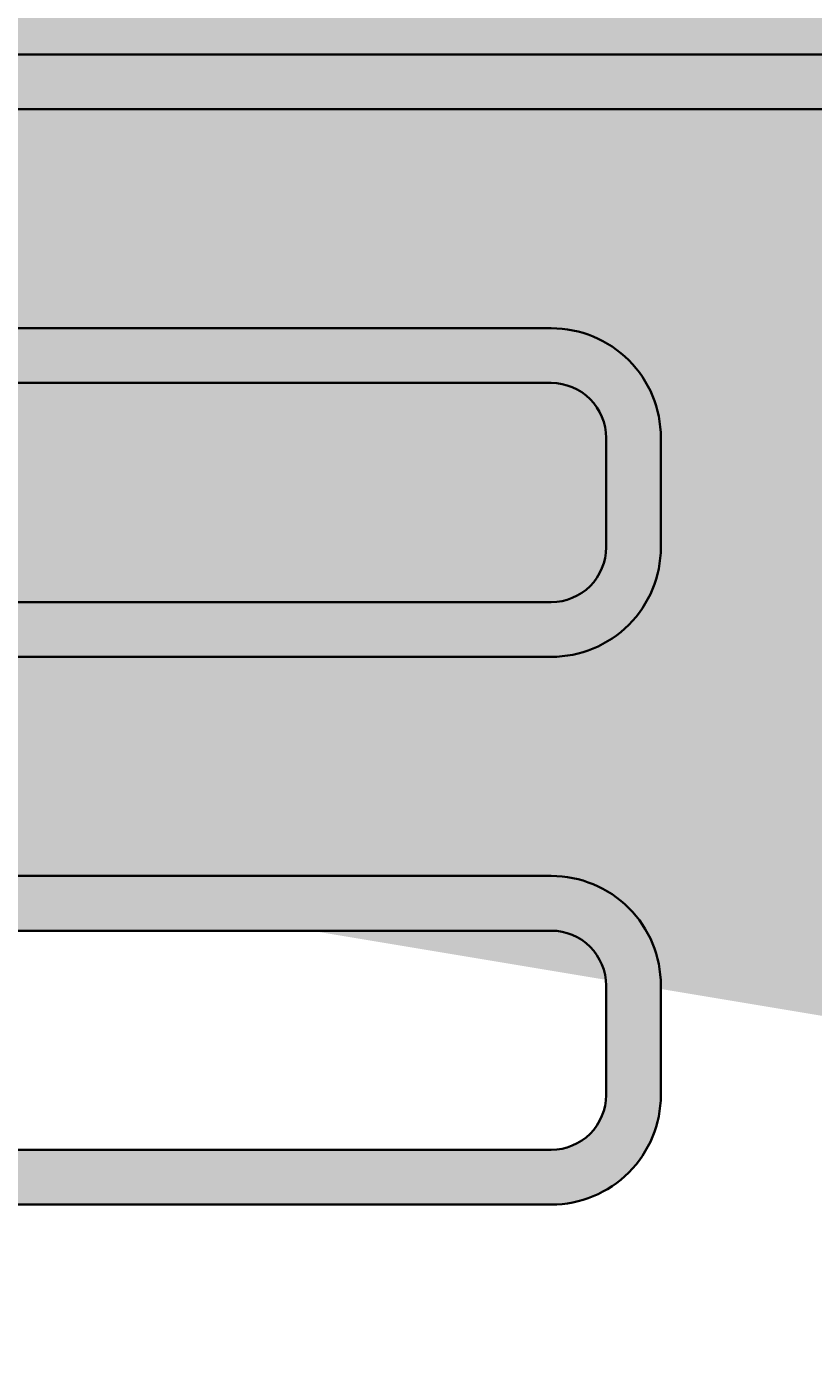
# Model space of a CAD drawing. Units: millimetres. Extents: x -22994 to 29398, y -19990 to 20176.
# Tile 40 of 135: x 169 to 183, y 54 to 78. Entities that reach past the tile are written whole.
import ezdxf

# ---------------------------------------------------------------- set-up
doc = ezdxf.new("R2010")
doc.units = ezdxf.units.MM
doc.header["$MEASUREMENT"] = 0
for name, color, linetype, lineweight in [('M-DIMS', 2, 'Continuous', 18), ('M-EQPM-PATT', 7, 'Continuous', 18), ('M-PIPE', 7, 'Continuous', 35)]:
    doc.layers.add(name, color=color, linetype=linetype, lineweight=lineweight)
doc.styles.get("Standard").update_dxf_attribs({"font": 'arial.ttf'})
doc.dimstyles.get("Standard").update_dxf_attribs({"dimtxt": 0.18, "dimasz": 10000, "dimexe": 0.18, "dimexo": 0.0625, "dimgap": 0.09, "dimtad": 0, "dimtih": 1, "dimtoh": 1, "dimdec": 0, "dimzin": 0, "dimdsep": 46, "dimtxsty": 'Standard', "dimcen": 0.09, "dimadec": 0, "dimazin": 0, "dimtfac": 1, "dimtdec": 0, "dimtofl": 0, "dimtmove": 0, "dimatfit": 3, "dimfxl": 1, "dimtolj": 1, "dimtzin": 0, "dimlwd": 30, "dimarcsym": 0})

# ---------------------------------------------------------------- blocks, each defined once
blk = doc.blocks.new('*D2')
at = {"layer": 'Defpoints', "color": 0, "transparency": 16777216}
for p in [(6.677, 10.271), (290.852, 10.271), (290.852, -5.079)]:
    blk.add_point(p, dxfattribs=at)
at = {"layer": 'M-DIMS', "color": 0, "lineweight": -2, "transparency": 16777216}
for p, q in [((6.677, 10.209), (6.677, -5.259)), ((290.852, 10.209), (290.852, -5.259))]:
    blk.add_line(p, q, dxfattribs=at)
at = {"layer": 'M-DIMS', "color": 0, "lineweight": 30, "transparency": 16777216}
for p, q in [((-9993.323, -5.079), (-19993.323, -5.079)), ((10290.852, -5.079), (20290.852, -5.079))]:
    blk.add_line(p, q, dxfattribs=at)
at = {"layer": 'M-DIMS', "color": 0, "transparency": 16777216}
for points in [[(-9993.323, 1661.588), (-9993.323, -1671.745), (6.677, -5.079)], [(10290.852, 1661.588), (10290.852, -1671.745), (290.852, -5.079)]]:
    blk.add_solid(points, dxfattribs=at)
at = {"layer": 'M-DIMS', "color": 0, "transparency": 16777216, "insert": (148.765, -5.079), "char_height": 0.18, "attachment_point": 5}
blk.add_mtext('\\A1;284.2', dxfattribs=at)
blk = doc.blocks.new('*D3')
at = {"layer": 'Defpoints', "color": 0, "transparency": 16777216}
for p in [(110.265, 204.165), (110.265, 176.366), (95.833, 127.967)]:
    blk.add_point(p, dxfattribs=at)
at = {"layer": 'M-DIMS', "color": 0, "lineweight": -2, "transparency": 16777216}
for p, q in [((95.833, 128.03), (95.833, 204.345)), ((110.265, 176.429), (110.265, 204.345))]:
    blk.add_line(p, q, dxfattribs=at)
at = {"layer": 'M-DIMS', "color": 0, "lineweight": 30, "transparency": 16777216}
for p, q in [((-9904.167, 204.165), (-19904.167, 204.165)), ((10110.265, 204.165), (20110.265, 204.165))]:
    blk.add_line(p, q, dxfattribs=at)
at = {"layer": 'M-DIMS', "color": 0, "transparency": 16777216}
for points in [[(-9904.167, 1870.832), (-9904.167, -1462.501), (95.833, 204.165)], [(10110.265, 1870.832), (10110.265, -1462.501), (110.265, 204.165)]]:
    blk.add_solid(points, dxfattribs=at)
at = {"layer": 'M-DIMS', "color": 0, "transparency": 16777216, "insert": (103.049, 204.165), "char_height": 0.18, "attachment_point": 5}
blk.add_mtext('\\A1;14.432', dxfattribs=at)
blk = doc.blocks.new('*D4')
at = {"layer": 'Defpoints', "color": 0, "transparency": 16777216}
for p in [(116.265, 204.165), (110.265, 176.366), (116.265, 176.366)]:
    blk.add_point(p, dxfattribs=at)
at = {"layer": 'M-DIMS', "color": 0, "lineweight": -2, "transparency": 16777216}
for p, q in [((110.265, 176.429), (110.265, 204.345)), ((116.265, 176.429), (116.265, 204.345))]:
    blk.add_line(p, q, dxfattribs=at)
at = {"layer": 'M-DIMS', "color": 0, "lineweight": 30, "transparency": 16777216}
for p, q in [((-9889.735, 204.165), (-19889.735, 204.165)), ((10116.265, 204.165), (20116.265, 204.165))]:
    blk.add_line(p, q, dxfattribs=at)
at = {"layer": 'M-DIMS', "color": 0, "transparency": 16777216}
for points in [[(-9889.735, 1870.832), (-9889.735, -1462.501), (110.265, 204.165)], [(10116.265, 1870.832), (10116.265, -1462.501), (116.265, 204.165)]]:
    blk.add_solid(points, dxfattribs=at)
at = {"layer": 'M-DIMS', "color": 0, "transparency": 16777216, "insert": (113.265, 204.165), "char_height": 0.18, "attachment_point": 5}
blk.add_mtext('\\A1;6', dxfattribs=at)
blk = doc.blocks.new('*D5')
at = {"layer": 'Defpoints', "color": 0, "transparency": 16777216}
for p in [(181.265, 204.165), (116.265, 176.366), (181.265, 176.366)]:
    blk.add_point(p, dxfattribs=at)
at = {"layer": 'M-DIMS', "color": 0, "lineweight": -2, "transparency": 16777216}
for p, q in [((116.265, 176.429), (116.265, 204.345)), ((181.265, 176.429), (181.265, 204.345))]:
    blk.add_line(p, q, dxfattribs=at)
at = {"layer": 'M-DIMS', "color": 0, "lineweight": 30, "transparency": 16777216}
for p, q in [((-9883.735, 204.165), (-19883.735, 204.165)), ((10181.265, 204.165), (20181.265, 204.165))]:
    blk.add_line(p, q, dxfattribs=at)
at = {"layer": 'M-DIMS', "color": 0, "transparency": 16777216}
for points in [[(-9883.735, 1870.832), (-9883.735, -1462.501), (116.265, 204.165)], [(10181.265, 1870.832), (10181.265, -1462.501), (181.265, 204.165)]]:
    blk.add_solid(points, dxfattribs=at)
at = {"layer": 'M-DIMS', "color": 0, "transparency": 16777216, "insert": (148.765, 204.165), "char_height": 0.18, "attachment_point": 5}
blk.add_mtext('\\A1;65', dxfattribs=at)
blk = doc.blocks.new('*D6')
at = {"layer": 'Defpoints', "color": 0, "transparency": 16777216}
for p in [(187.265, 204.165), (181.265, 176.366), (187.265, 176.366)]:
    blk.add_point(p, dxfattribs=at)
at = {"layer": 'M-DIMS', "color": 0, "lineweight": -2, "transparency": 16777216}
for p, q in [((181.265, 176.429), (181.265, 204.345)), ((187.265, 176.429), (187.265, 204.345))]:
    blk.add_line(p, q, dxfattribs=at)
at = {"layer": 'M-DIMS', "color": 0, "lineweight": 30, "transparency": 16777216}
for p, q in [((-9818.735, 204.165), (-19818.735, 204.165)), ((10187.265, 204.165), (20187.265, 204.165))]:
    blk.add_line(p, q, dxfattribs=at)
at = {"layer": 'M-DIMS', "color": 0, "transparency": 16777216}
for points in [[(-9818.735, 1870.832), (-9818.735, -1462.501), (181.265, 204.165)], [(10187.265, 1870.832), (10187.265, -1462.501), (187.265, 204.165)]]:
    blk.add_solid(points, dxfattribs=at)
at = {"layer": 'M-DIMS', "color": 0, "transparency": 16777216, "insert": (184.265, 204.165), "char_height": 0.18, "attachment_point": 5}
blk.add_mtext('\\A1;6', dxfattribs=at)
blk = doc.blocks.new('*D7')
at = {"layer": 'Defpoints', "color": 0, "transparency": 16777216}
for p in [(201.697, 204.165), (187.265, 176.366), (201.697, 127.967)]:
    blk.add_point(p, dxfattribs=at)
at = {"layer": 'M-DIMS', "color": 0, "lineweight": -2, "transparency": 16777216}
for p, q in [((187.265, 176.429), (187.265, 204.345)), ((201.697, 128.03), (201.697, 204.345))]:
    blk.add_line(p, q, dxfattribs=at)
at = {"layer": 'M-DIMS', "color": 0, "lineweight": 30, "transparency": 16777216}
for p, q in [((-9812.735, 204.165), (-19812.735, 204.165)), ((10201.697, 204.165), (20201.697, 204.165))]:
    blk.add_line(p, q, dxfattribs=at)
at = {"layer": 'M-DIMS', "color": 0, "transparency": 16777216}
for points in [[(-9812.735, 1870.832), (-9812.735, -1462.501), (187.265, 204.165)], [(10201.697, 1870.832), (10201.697, -1462.501), (201.697, 204.165)]]:
    blk.add_solid(points, dxfattribs=at)
at = {"layer": 'M-DIMS', "color": 0, "transparency": 16777216, "insert": (194.481, 204.165), "char_height": 0.18, "attachment_point": 5}
blk.add_mtext('\\A1;14.432', dxfattribs=at)
blk = doc.blocks.new('*D8')
at = {"layer": 'Defpoints', "color": 0, "transparency": 16777216}
for p in [(227.648, 204.165), (227.648, 146.73), (201.697, 127.967)]:
    blk.add_point(p, dxfattribs=at)
at = {"layer": 'M-DIMS', "color": 0, "lineweight": -2, "transparency": 16777216}
for p, q in [((201.697, 128.03), (201.697, 204.345)), ((227.648, 146.792), (227.648, 204.345))]:
    blk.add_line(p, q, dxfattribs=at)
at = {"layer": 'M-DIMS', "color": 0, "lineweight": 30, "transparency": 16777216}
for p, q in [((-9798.303, 204.165), (-19798.303, 204.165)), ((10227.648, 204.165), (20227.648, 204.165))]:
    blk.add_line(p, q, dxfattribs=at)
at = {"layer": 'M-DIMS', "color": 0, "transparency": 16777216}
for points in [[(-9798.303, 1870.832), (-9798.303, -1462.501), (201.697, 204.165)], [(10227.648, 1870.832), (10227.648, -1462.501), (227.648, 204.165)]]:
    blk.add_solid(points, dxfattribs=at)
at = {"layer": 'M-DIMS', "color": 0, "transparency": 16777216, "insert": (214.673, 204.165), "char_height": 0.18, "attachment_point": 5}
blk.add_mtext('\\A1;25.95', dxfattribs=at)
blk = doc.blocks.new('*D9')
at = {"layer": 'Defpoints', "color": 0, "transparency": 16777216}
for p in [(187.265, 176.366), (306.202, 176.366), (290.852, 10.271)]:
    blk.add_point(p, dxfattribs=at)
at = {"layer": 'M-DIMS', "color": 0, "lineweight": 30, "transparency": 16777216}
for p, q in [((306.202, 10176.366), (306.202, 20176.366)), ((306.202, -9989.729), (306.202, -19989.729))]:
    blk.add_line(p, q, dxfattribs=at)
at = {"layer": 'M-DIMS', "color": 0, "lineweight": -2, "transparency": 16777216}
for p, q in [((187.327, 176.366), (306.382, 176.366)), ((290.915, 10.271), (306.382, 10.271))]:
    blk.add_line(p, q, dxfattribs=at)
at = {"layer": 'M-DIMS', "color": 0, "transparency": 16777216}
for points in [[(-1360.465, 10176.366), (1972.869, 10176.366), (306.202, 176.366)], [(-1360.465, -9989.729), (1972.869, -9989.729), (306.202, 10.271)]]:
    blk.add_solid(points, dxfattribs=at)
at = {"layer": 'M-DIMS', "color": 0, "transparency": 16777216, "insert": (306.202, 93.319), "char_height": 0.18, "attachment_point": 5}
blk.add_mtext('\\A1;166.1', dxfattribs=at)
blk = doc.blocks.new('*D10')
at = {"layer": 'Defpoints', "color": 0, "transparency": 16777216}
for p in [(125.65, 136.071), (133.346, 136.071), (133.346, -5.079)]:
    blk.add_point(p, dxfattribs=at)
at = {"layer": 'M-DIMS', "color": 0, "lineweight": -2, "transparency": 16777216}
for p, q in [((125.65, 136.009), (125.65, -5.259)), ((133.346, 136.009), (133.346, -5.259))]:
    blk.add_line(p, q, dxfattribs=at)
at = {"layer": 'M-DIMS', "color": 0, "lineweight": 30, "transparency": 16777216}
for p, q in [((-9874.35, -5.079), (-19874.35, -5.079)), ((10133.346, -5.079), (20133.346, -5.079))]:
    blk.add_line(p, q, dxfattribs=at)
at = {"layer": 'M-DIMS', "color": 0, "transparency": 16777216}
for points in [[(-9874.35, 1661.588), (-9874.35, -1671.745), (125.65, -5.079)], [(10133.346, 1661.588), (10133.346, -1671.745), (133.346, -5.079)]]:
    blk.add_solid(points, dxfattribs=at)
at = {"layer": 'M-DIMS', "color": 0, "transparency": 16777216, "insert": (129.498, -5.079), "char_height": 0.18, "attachment_point": 5}
blk.add_mtext('\\A1;7.696', dxfattribs=at)
blk = doc.blocks.new('*D11')
at = {"layer": 'Defpoints', "color": 0, "transparency": 16777216}
for p in [(133.346, 136.071), (135.65, 136.071), (135.65, -5.079)]:
    blk.add_point(p, dxfattribs=at)
at = {"layer": 'M-DIMS', "color": 0, "lineweight": -2, "transparency": 16777216}
for p, q in [((133.346, 136.009), (133.346, -5.259)), ((135.65, 136.009), (135.65, -5.259))]:
    blk.add_line(p, q, dxfattribs=at)
at = {"layer": 'M-DIMS', "color": 0, "lineweight": 30, "transparency": 16777216}
for p, q in [((-9866.654, -5.079), (-19866.654, -5.079)), ((10135.65, -5.079), (20135.65, -5.079))]:
    blk.add_line(p, q, dxfattribs=at)
at = {"layer": 'M-DIMS', "color": 0, "transparency": 16777216}
for points in [[(-9866.654, 1661.588), (-9866.654, -1671.745), (133.346, -5.079)], [(10135.65, 1661.588), (10135.65, -1671.745), (135.65, -5.079)]]:
    blk.add_solid(points, dxfattribs=at)
at = {"layer": 'M-DIMS', "color": 0, "transparency": 16777216, "insert": (134.498, -5.079), "char_height": 0.18, "attachment_point": 5}
blk.add_mtext('\\A1;2.304', dxfattribs=at)
blk = doc.blocks.new('*D12')
at = {"layer": 'Defpoints', "color": 0, "transparency": 16777216}
for p in [(135.65, 136.071), (145.65, 136.071), (145.65, -5.079)]:
    blk.add_point(p, dxfattribs=at)
at = {"layer": 'M-DIMS', "color": 0, "lineweight": -2, "transparency": 16777216}
for p, q in [((135.65, 136.009), (135.65, -5.259)), ((145.65, 136.009), (145.65, -5.259))]:
    blk.add_line(p, q, dxfattribs=at)
at = {"layer": 'M-DIMS', "color": 0, "lineweight": 30, "transparency": 16777216}
for p, q in [((-9864.35, -5.079), (-19864.35, -5.079)), ((10145.65, -5.079), (20145.65, -5.079))]:
    blk.add_line(p, q, dxfattribs=at)
at = {"layer": 'M-DIMS', "color": 0, "transparency": 16777216}
for points in [[(-9864.35, 1661.588), (-9864.35, -1671.745), (135.65, -5.079)], [(10145.65, 1661.588), (10145.65, -1671.745), (145.65, -5.079)]]:
    blk.add_solid(points, dxfattribs=at)
at = {"layer": 'M-DIMS', "color": 0, "transparency": 16777216, "insert": (140.65, -5.079), "char_height": 0.18, "attachment_point": 5}
blk.add_mtext('\\A1;10', dxfattribs=at)
blk = doc.blocks.new('*D13')
at = {"layer": 'Defpoints', "color": 0, "transparency": 16777216}
for p in [(145.65, 136.071), (155.65, 136.071), (155.65, -5.079)]:
    blk.add_point(p, dxfattribs=at)
at = {"layer": 'M-DIMS', "color": 0, "lineweight": -2, "transparency": 16777216}
for p, q in [((145.65, 136.009), (145.65, -5.259)), ((155.65, 136.009), (155.65, -5.259))]:
    blk.add_line(p, q, dxfattribs=at)
at = {"layer": 'M-DIMS', "color": 0, "lineweight": 30, "transparency": 16777216}
for p, q in [((-9854.35, -5.079), (-19854.35, -5.079)), ((10155.65, -5.079), (20155.65, -5.079))]:
    blk.add_line(p, q, dxfattribs=at)
at = {"layer": 'M-DIMS', "color": 0, "transparency": 16777216}
for points in [[(-9854.35, 1661.588), (-9854.35, -1671.745), (145.65, -5.079)], [(10155.65, 1661.588), (10155.65, -1671.745), (155.65, -5.079)]]:
    blk.add_solid(points, dxfattribs=at)
at = {"layer": 'M-DIMS', "color": 0, "transparency": 16777216, "insert": (150.65, -5.079), "char_height": 0.18, "attachment_point": 5}
blk.add_mtext('\\A1;10', dxfattribs=at)
blk = doc.blocks.new('*D14')
at = {"layer": 'Defpoints', "color": 0, "transparency": 16777216}
for p in [(155.65, 136.071), (165.65, 136.071), (165.65, -5.079)]:
    blk.add_point(p, dxfattribs=at)
at = {"layer": 'M-DIMS', "color": 0, "lineweight": -2, "transparency": 16777216}
for p, q in [((155.65, 136.009), (155.65, -5.259)), ((165.65, 136.009), (165.65, -5.259))]:
    blk.add_line(p, q, dxfattribs=at)
at = {"layer": 'M-DIMS', "color": 0, "lineweight": 30, "transparency": 16777216}
for p, q in [((-9844.35, -5.079), (-19844.35, -5.079)), ((10165.65, -5.079), (20165.65, -5.079))]:
    blk.add_line(p, q, dxfattribs=at)
at = {"layer": 'M-DIMS', "color": 0, "transparency": 16777216}
for points in [[(-9844.35, 1661.588), (-9844.35, -1671.745), (155.65, -5.079)], [(10165.65, 1661.588), (10165.65, -1671.745), (165.65, -5.079)]]:
    blk.add_solid(points, dxfattribs=at)
at = {"layer": 'M-DIMS', "color": 0, "transparency": 16777216, "insert": (160.65, -5.079), "char_height": 0.18, "attachment_point": 5}
blk.add_mtext('\\A1;10', dxfattribs=at)
blk = doc.blocks.new('*D15')
at = {"layer": 'Defpoints', "color": 0, "transparency": 16777216}
for p in [(173.346, 154.788), (173.346, 136.071), (306.202, 136.071)]:
    blk.add_point(p, dxfattribs=at)
at = {"layer": 'M-DIMS', "color": 0, "lineweight": 30, "transparency": 16777216}
for p, q in [((306.202, 10154.788), (306.202, 20154.788)), ((306.202, -9863.929), (306.202, -19863.929))]:
    blk.add_line(p, q, dxfattribs=at)
at = {"layer": 'M-DIMS', "color": 0, "lineweight": -2, "transparency": 16777216}
for p, q in [((173.408, 154.788), (306.382, 154.788)), ((173.408, 136.071), (306.382, 136.071))]:
    blk.add_line(p, q, dxfattribs=at)
at = {"layer": 'M-DIMS', "color": 0, "transparency": 16777216}
for points in [[(-1360.465, 10154.788), (1972.869, 10154.788), (306.202, 154.788)], [(-1360.465, -9863.929), (1972.869, -9863.929), (306.202, 136.071)]]:
    blk.add_solid(points, dxfattribs=at)
at = {"layer": 'M-DIMS', "color": 0, "transparency": 16777216, "insert": (306.202, 145.43), "char_height": 0.18, "attachment_point": 5}
blk.add_mtext('\\A1;18.717', dxfattribs=at)
blk = doc.blocks.new('*D16')
at = {"layer": 'Defpoints', "color": 0, "transparency": 16777216}
for p in [(120.17, 204.165), (110.466, 48.035), (120.17, 48.035)]:
    blk.add_point(p, dxfattribs=at)
at = {"layer": 'M-DIMS', "color": 0, "lineweight": -2, "transparency": 16777216}
for p, q in [((110.466, 48.097), (110.466, 204.345)), ((120.17, 48.097), (120.17, 204.345))]:
    blk.add_line(p, q, dxfattribs=at)
at = {"layer": 'M-DIMS', "color": 0, "lineweight": 30, "transparency": 16777216}
for p, q in [((-9889.534, 204.165), (-19889.534, 204.165)), ((10120.17, 204.165), (20120.17, 204.165))]:
    blk.add_line(p, q, dxfattribs=at)
at = {"layer": 'M-DIMS', "color": 0, "transparency": 16777216}
for points in [[(-9889.534, 1870.832), (-9889.534, -1462.501), (110.466, 204.165)], [(10120.17, 1870.832), (10120.17, -1462.501), (120.17, 204.165)]]:
    blk.add_solid(points, dxfattribs=at)
at = {"layer": 'M-DIMS', "color": 0, "transparency": 16777216, "insert": (115.318, 204.165), "char_height": 0.18, "attachment_point": 5}
blk.add_mtext('\\A1;9.704', dxfattribs=at)
blk = doc.blocks.new('*D17')
at = {"layer": 'Defpoints', "color": 0, "transparency": 16777216}
for p in [(126.17, 204.165), (120.17, 48.035), (126.17, 48.035)]:
    blk.add_point(p, dxfattribs=at)
at = {"layer": 'M-DIMS', "color": 0, "lineweight": -2, "transparency": 16777216}
for p, q in [((120.17, 48.097), (120.17, 204.345)), ((126.17, 48.097), (126.17, 204.345))]:
    blk.add_line(p, q, dxfattribs=at)
at = {"layer": 'M-DIMS', "color": 0, "lineweight": 30, "transparency": 16777216}
for p, q in [((-9879.83, 204.165), (-19879.83, 204.165)), ((10126.17, 204.165), (20126.17, 204.165))]:
    blk.add_line(p, q, dxfattribs=at)
at = {"layer": 'M-DIMS', "color": 0, "transparency": 16777216}
for points in [[(-9879.83, 1870.832), (-9879.83, -1462.501), (120.17, 204.165)], [(10126.17, 1870.832), (10126.17, -1462.501), (126.17, 204.165)]]:
    blk.add_solid(points, dxfattribs=at)
at = {"layer": 'M-DIMS', "color": 0, "transparency": 16777216, "insert": (123.17, 204.165), "char_height": 0.18, "attachment_point": 5}
blk.add_mtext('\\A1;6', dxfattribs=at)
blk = doc.blocks.new('*D18')
at = {"layer": 'Defpoints', "color": 0, "transparency": 16777216}
for p in [(132.17, 204.165), (126.17, 48.035), (132.17, 48.035)]:
    blk.add_point(p, dxfattribs=at)
at = {"layer": 'M-DIMS', "color": 0, "lineweight": -2, "transparency": 16777216}
for p, q in [((126.17, 48.097), (126.17, 204.345)), ((132.17, 48.097), (132.17, 204.345))]:
    blk.add_line(p, q, dxfattribs=at)
at = {"layer": 'M-DIMS', "color": 0, "lineweight": 30, "transparency": 16777216}
for p, q in [((-9873.83, 204.165), (-19873.83, 204.165)), ((10132.17, 204.165), (20132.17, 204.165))]:
    blk.add_line(p, q, dxfattribs=at)
at = {"layer": 'M-DIMS', "color": 0, "transparency": 16777216}
for points in [[(-9873.83, 1870.832), (-9873.83, -1462.501), (126.17, 204.165)], [(10132.17, 1870.832), (10132.17, -1462.501), (132.17, 204.165)]]:
    blk.add_solid(points, dxfattribs=at)
at = {"layer": 'M-DIMS', "color": 0, "transparency": 16777216, "insert": (129.17, 204.165), "char_height": 0.18, "attachment_point": 5}
blk.add_mtext('\\A1;6', dxfattribs=at)
blk = doc.blocks.new('*D19')
at = {"layer": 'Defpoints', "color": 0, "transparency": 16777216}
for p in [(138.17, 204.165), (132.17, 48.035), (138.17, 48.035)]:
    blk.add_point(p, dxfattribs=at)
at = {"layer": 'M-DIMS', "color": 0, "lineweight": -2, "transparency": 16777216}
for p, q in [((132.17, 48.097), (132.17, 204.345)), ((138.17, 48.097), (138.17, 204.345))]:
    blk.add_line(p, q, dxfattribs=at)
at = {"layer": 'M-DIMS', "color": 0, "lineweight": 30, "transparency": 16777216}
for p, q in [((-9867.83, 204.165), (-19867.83, 204.165)), ((10138.17, 204.165), (20138.17, 204.165))]:
    blk.add_line(p, q, dxfattribs=at)
at = {"layer": 'M-DIMS', "color": 0, "transparency": 16777216}
for points in [[(-9867.83, 1870.832), (-9867.83, -1462.501), (132.17, 204.165)], [(10138.17, 1870.832), (10138.17, -1462.501), (138.17, 204.165)]]:
    blk.add_solid(points, dxfattribs=at)
at = {"layer": 'M-DIMS', "color": 0, "transparency": 16777216, "insert": (135.17, 204.165), "char_height": 0.18, "attachment_point": 5}
blk.add_mtext('\\A1;6', dxfattribs=at)
blk = doc.blocks.new('*D20')
at = {"layer": 'Defpoints', "color": 0, "transparency": 16777216}
for p in [(144.17, 204.165), (138.17, 48.035), (144.17, 48.035)]:
    blk.add_point(p, dxfattribs=at)
at = {"layer": 'M-DIMS', "color": 0, "lineweight": -2, "transparency": 16777216}
for p, q in [((138.17, 48.097), (138.17, 204.345)), ((144.17, 48.097), (144.17, 204.345))]:
    blk.add_line(p, q, dxfattribs=at)
at = {"layer": 'M-DIMS', "color": 0, "lineweight": 30, "transparency": 16777216}
for p, q in [((-9861.83, 204.165), (-19861.83, 204.165)), ((10144.17, 204.165), (20144.17, 204.165))]:
    blk.add_line(p, q, dxfattribs=at)
at = {"layer": 'M-DIMS', "color": 0, "transparency": 16777216}
for points in [[(-9861.83, 1870.832), (-9861.83, -1462.501), (138.17, 204.165)], [(10144.17, 1870.832), (10144.17, -1462.501), (144.17, 204.165)]]:
    blk.add_solid(points, dxfattribs=at)
at = {"layer": 'M-DIMS', "color": 0, "transparency": 16777216, "insert": (141.17, 204.165), "char_height": 0.18, "attachment_point": 5}
blk.add_mtext('\\A1;6', dxfattribs=at)
blk = doc.blocks.new('*D21')
at = {"layer": 'Defpoints', "color": 0, "transparency": 16777216}
for p in [(149.116, 204.165), (144.17, 48.035), (149.116, 48.035)]:
    blk.add_point(p, dxfattribs=at)
at = {"layer": 'M-DIMS', "color": 0, "lineweight": -2, "transparency": 16777216}
for p, q in [((144.17, 48.097), (144.17, 204.345)), ((149.116, 48.097), (149.116, 204.345))]:
    blk.add_line(p, q, dxfattribs=at)
at = {"layer": 'M-DIMS', "color": 0, "lineweight": 30, "transparency": 16777216}
for p, q in [((-9855.83, 204.165), (-19855.83, 204.165)), ((10149.116, 204.165), (20149.116, 204.165))]:
    blk.add_line(p, q, dxfattribs=at)
at = {"layer": 'M-DIMS', "color": 0, "transparency": 16777216}
for points in [[(-9855.83, 1870.832), (-9855.83, -1462.501), (144.17, 204.165)], [(10149.116, 1870.832), (10149.116, -1462.501), (149.116, 204.165)]]:
    blk.add_solid(points, dxfattribs=at)
at = {"layer": 'M-DIMS', "color": 0, "transparency": 16777216, "insert": (146.643, 204.165), "char_height": 0.18, "attachment_point": 5}
blk.add_mtext('\\A1;4.945', dxfattribs=at)
blk = doc.blocks.new('*D22')
at = {"layer": 'Defpoints', "color": 0, "transparency": 16777216}
for p in [(149.116, 30.99), (155.116, 30.99), (155.116, -5.079)]:
    blk.add_point(p, dxfattribs=at)
at = {"layer": 'M-DIMS', "color": 0, "lineweight": -2, "transparency": 16777216}
for p, q in [((149.116, 30.927), (149.116, -5.259)), ((155.116, 30.927), (155.116, -5.259))]:
    blk.add_line(p, q, dxfattribs=at)
at = {"layer": 'M-DIMS', "color": 0, "lineweight": 30, "transparency": 16777216}
for p, q in [((-9850.884, -5.079), (-19850.884, -5.079)), ((10155.116, -5.079), (20155.116, -5.079))]:
    blk.add_line(p, q, dxfattribs=at)
at = {"layer": 'M-DIMS', "color": 0, "transparency": 16777216}
for points in [[(-9850.884, 1661.588), (-9850.884, -1671.745), (149.116, -5.079)], [(10155.116, 1661.588), (10155.116, -1671.745), (155.116, -5.079)]]:
    blk.add_solid(points, dxfattribs=at)
at = {"layer": 'M-DIMS', "color": 0, "transparency": 16777216, "insert": (152.116, -5.079), "char_height": 0.18, "attachment_point": 5}
blk.add_mtext('\\A1;6', dxfattribs=at)
blk = doc.blocks.new('*D23')
at = {"layer": 'Defpoints', "color": 0, "transparency": 16777216}
for p in [(155.116, 30.99), (161.116, 30.99), (161.116, -5.079)]:
    blk.add_point(p, dxfattribs=at)
at = {"layer": 'M-DIMS', "color": 0, "lineweight": -2, "transparency": 16777216}
for p, q in [((155.116, 30.927), (155.116, -5.259)), ((161.116, 30.927), (161.116, -5.259))]:
    blk.add_line(p, q, dxfattribs=at)
at = {"layer": 'M-DIMS', "color": 0, "lineweight": 30, "transparency": 16777216}
for p, q in [((-9844.884, -5.079), (-19844.884, -5.079)), ((10161.116, -5.079), (20161.116, -5.079))]:
    blk.add_line(p, q, dxfattribs=at)
at = {"layer": 'M-DIMS', "color": 0, "transparency": 16777216}
for points in [[(-9844.884, 1661.588), (-9844.884, -1671.745), (155.116, -5.079)], [(10161.116, 1661.588), (10161.116, -1671.745), (161.116, -5.079)]]:
    blk.add_solid(points, dxfattribs=at)
at = {"layer": 'M-DIMS', "color": 0, "transparency": 16777216, "insert": (158.116, -5.079), "char_height": 0.18, "attachment_point": 5}
blk.add_mtext('\\A1;6', dxfattribs=at)
blk = doc.blocks.new('*D24')
at = {"layer": 'Defpoints', "color": 0, "transparency": 16777216}
for p in [(161.116, 30.99), (166.439, 30.99), (166.439, -5.079)]:
    blk.add_point(p, dxfattribs=at)
at = {"layer": 'M-DIMS', "color": 0, "lineweight": -2, "transparency": 16777216}
for p, q in [((161.116, 30.927), (161.116, -5.259)), ((166.439, 30.927), (166.439, -5.259))]:
    blk.add_line(p, q, dxfattribs=at)
at = {"layer": 'M-DIMS', "color": 0, "lineweight": 30, "transparency": 16777216}
for p, q in [((-9838.884, -5.079), (-19838.884, -5.079)), ((10166.439, -5.079), (20166.439, -5.079))]:
    blk.add_line(p, q, dxfattribs=at)
at = {"layer": 'M-DIMS', "color": 0, "transparency": 16777216}
for points in [[(-9838.884, 1661.588), (-9838.884, -1671.745), (161.116, -5.079)], [(10166.439, 1661.588), (10166.439, -1671.745), (166.439, -5.079)]]:
    blk.add_solid(points, dxfattribs=at)
at = {"layer": 'M-DIMS', "color": 0, "transparency": 16777216, "insert": (163.777, -5.079), "char_height": 0.18, "attachment_point": 5}
blk.add_mtext('\\A1;5.323', dxfattribs=at)
blk = doc.blocks.new('*D25')
at = {"layer": 'Defpoints', "color": 0, "transparency": 16777216}
for p in [(166.439, 30.99), (172.439, 30.99), (172.439, -5.079)]:
    blk.add_point(p, dxfattribs=at)
at = {"layer": 'M-DIMS', "color": 0, "lineweight": -2, "transparency": 16777216}
for p, q in [((166.439, 30.927), (166.439, -5.259)), ((172.439, 30.927), (172.439, -5.259))]:
    blk.add_line(p, q, dxfattribs=at)
at = {"layer": 'M-DIMS', "color": 0, "lineweight": 30, "transparency": 16777216}
for p, q in [((-9833.561, -5.079), (-19833.561, -5.079)), ((10172.439, -5.079), (20172.439, -5.079))]:
    blk.add_line(p, q, dxfattribs=at)
at = {"layer": 'M-DIMS', "color": 0, "transparency": 16777216}
for points in [[(-9833.561, 1661.588), (-9833.561, -1671.745), (166.439, -5.079)], [(10172.439, 1661.588), (10172.439, -1671.745), (172.439, -5.079)]]:
    blk.add_solid(points, dxfattribs=at)
at = {"layer": 'M-DIMS', "color": 0, "transparency": 16777216, "insert": (169.439, -5.079), "char_height": 0.18, "attachment_point": 5}
blk.add_mtext('\\A1;6', dxfattribs=at)
blk = doc.blocks.new('*D26')
at = {"layer": 'Defpoints', "color": 0, "transparency": 16777216}
for p in [(172.439, 30.99), (178.439, 30.99), (178.439, -5.079)]:
    blk.add_point(p, dxfattribs=at)
at = {"layer": 'M-DIMS', "color": 0, "lineweight": -2, "transparency": 16777216}
for p, q in [((172.439, 30.927), (172.439, -5.259)), ((178.439, 30.927), (178.439, -5.259))]:
    blk.add_line(p, q, dxfattribs=at)
at = {"layer": 'M-DIMS', "color": 0, "lineweight": 30, "transparency": 16777216}
for p, q in [((-9827.561, -5.079), (-19827.561, -5.079)), ((10178.439, -5.079), (20178.439, -5.079))]:
    blk.add_line(p, q, dxfattribs=at)
at = {"layer": 'M-DIMS', "color": 0, "transparency": 16777216}
for points in [[(-9827.561, 1661.588), (-9827.561, -1671.745), (172.439, -5.079)], [(10178.439, 1661.588), (10178.439, -1671.745), (178.439, -5.079)]]:
    blk.add_solid(points, dxfattribs=at)
at = {"layer": 'M-DIMS', "color": 0, "transparency": 16777216, "insert": (175.439, -5.079), "char_height": 0.18, "attachment_point": 5}
blk.add_mtext('\\A1;6', dxfattribs=at)
blk = doc.blocks.new('*D27')
at = {"layer": 'Defpoints', "color": 0, "transparency": 16777216}
for p in [(178.439, 30.99), (188.117, 30.99), (188.117, -5.079)]:
    blk.add_point(p, dxfattribs=at)
at = {"layer": 'M-DIMS', "color": 0, "lineweight": -2, "transparency": 16777216}
for p, q in [((178.439, 30.927), (178.439, -5.259)), ((188.117, 30.927), (188.117, -5.259))]:
    blk.add_line(p, q, dxfattribs=at)
at = {"layer": 'M-DIMS', "color": 0, "lineweight": 30, "transparency": 16777216}
for p, q in [((-9821.561, -5.079), (-19821.561, -5.079)), ((10188.117, -5.079), (20188.117, -5.079))]:
    blk.add_line(p, q, dxfattribs=at)
at = {"layer": 'M-DIMS', "color": 0, "transparency": 16777216}
for points in [[(-9821.561, 1661.588), (-9821.561, -1671.745), (178.439, -5.079)], [(10188.117, 1661.588), (10188.117, -1671.745), (188.117, -5.079)]]:
    blk.add_solid(points, dxfattribs=at)
at = {"layer": 'M-DIMS', "color": 0, "transparency": 16777216, "insert": (183.278, -5.079), "char_height": 0.18, "attachment_point": 5}
blk.add_mtext('\\A1;9.679', dxfattribs=at)
blk = doc.blocks.new('*D28')
at = {"layer": 'Defpoints', "color": 0, "transparency": 16777216}
for p in [(188.117, 48.035), (306.202, 48.035), (188.117, 30.99)]:
    blk.add_point(p, dxfattribs=at)
at = {"layer": 'M-DIMS', "color": 0, "lineweight": 30, "transparency": 16777216}
for p, q in [((306.202, 10048.035), (306.202, 20048.035)), ((306.202, -9969.01), (306.202, -19969.01))]:
    blk.add_line(p, q, dxfattribs=at)
at = {"layer": 'M-DIMS', "color": 0, "lineweight": -2, "transparency": 16777216}
for p, q in [((188.18, 48.035), (306.382, 48.035)), ((188.18, 30.99), (306.382, 30.99))]:
    blk.add_line(p, q, dxfattribs=at)
at = {"layer": 'M-DIMS', "color": 0, "transparency": 16777216}
for points in [[(-1360.465, 10048.035), (1972.869, 10048.035), (306.202, 48.035)], [(-1360.465, -9969.01), (1972.869, -9969.01), (306.202, 30.99)]]:
    blk.add_solid(points, dxfattribs=at)
at = {"layer": 'M-DIMS', "color": 0, "transparency": 16777216, "insert": (306.202, 39.512), "char_height": 0.18, "attachment_point": 5}
blk.add_mtext('\\A1;17.045', dxfattribs=at)
blk = doc.blocks.new('*D29')
at = {"layer": 'Defpoints', "color": 0, "transparency": 16777216}
for p in [(36.801, 80.045), (64.03, 80.045)]:
    blk.add_point(p, dxfattribs=at)
at = {"layer": 'M-DIMS', "color": 0, "lineweight": -2, "transparency": 16777216}
for p, q in [((50.325, 80.045), (50.505, 80.045)), ((50.415, 79.955), (50.415, 80.135))]:
    blk.add_line(p, q, dxfattribs=at)
at = {"layer": 'M-DIMS', "color": 0, "lineweight": 30, "transparency": 16777216}
blk.add_line((20064.03, 80.03), (10064.03, 80.038), dxfattribs=at)
at = {"layer": 'M-DIMS', "color": 0, "transparency": 16777216}
blk.add_solid([(10064.031, 1746.704), (10064.028, -1586.629), (64.03, 80.045)], dxfattribs=at)
at = {"layer": 'M-DIMS', "color": 0, "transparency": 16777216, "insert": (20064.521, 80.03), "char_height": 0.18, "attachment_point": 5}
blk.add_mtext('\\A1;∅27.23', dxfattribs=at)
blk = doc.blocks.new('*D36')
at = {"layer": 'Defpoints', "color": 0, "transparency": 16777216}
for p in [(46.39, 31.303), (46.387, 26.593)]:
    blk.add_point(p, dxfattribs=at)
at = {"layer": 'M-DIMS', "color": 0, "lineweight": 30, "transparency": 16777216}
for p, q in [((57.15, 20031.301), (51.77, 10031.302)), ((10057.15, 20031.301), (57.15, 20031.301))]:
    blk.add_line(p, q, dxfattribs=at)
at = {"layer": 'M-DIMS', "color": 0, "lineweight": -2, "transparency": 16777216}
for p, q in [((46.299, 28.948), (46.479, 28.948)), ((46.389, 28.858), (46.389, 29.038))]:
    blk.add_line(p, q, dxfattribs=at)
at = {"layer": 'M-DIMS', "color": 0, "transparency": 16777216}
blk.add_solid([(-1614.896, 10032.199), (1718.436, 10030.405), (46.39, 31.303)], dxfattribs=at)
at = {"layer": 'M-DIMS', "color": 0, "transparency": 16777216, "insert": (10057.554, 20031.301), "char_height": 0.18, "attachment_point": 5}
blk.add_mtext('\\A1;∅4.71', dxfattribs=at)
blk = doc.blocks.new('*D37')
at = {"layer": 'Defpoints', "color": 0, "transparency": 16777216}
for p in [(54.834, 118.615), (59.494, 118.614)]:
    blk.add_point(p, dxfattribs=at)
at = {"layer": 'M-DIMS', "color": 0, "lineweight": -2, "transparency": 16777216}
for p, q in [((57.074, 118.614), (57.254, 118.614)), ((57.164, 118.524), (57.164, 118.704))]:
    blk.add_line(p, q, dxfattribs=at)
at = {"layer": 'M-DIMS', "color": 0, "lineweight": 30, "transparency": 16777216}
blk.add_line((20059.493, 116.253), (10059.494, 117.434), dxfattribs=at)
at = {"layer": 'M-DIMS', "color": 0, "transparency": 16777216}
blk.add_solid([(10059.69, 1784.1), (10059.297, -1549.233), (59.494, 118.614)], dxfattribs=at)
at = {"layer": 'M-DIMS', "color": 0, "transparency": 16777216, "insert": (20059.985, 116.253), "char_height": 0.18, "attachment_point": 5}
blk.add_mtext('\\A1;∅4.659', dxfattribs=at)

msp = doc.modelspace()

# ---------------------------------------------------------------- hatches: boundary and pattern name
at = {"layer": 'M-EQPM-PATT'}
h = msp.add_hatch(color=256, dxfattribs=at)
h.set_gradient(color1=(19, 155, 72), color2=(88, 186, 72), tint=1, name='CYLINDER')
h.paths.add_polyline_path([(109.4658, 29.9895), (189.1175, 29.9895), (189.1175, 77.6953), (128.1172, 77.6953, 0.4142136), (126.1172, 75.6953), (126.1172, 73.6953, 0.4142136), (128.1172, 71.6953), (178.5136, 71.6953, -0.4142136), (179.5136, 70.6953), (179.5136, 68.6953, -0.4142136), (178.5136, 67.6953), (128.1172, 67.6953, 0.4142136), (126.1172, 65.6953), (126.1172, 63.6953, 0.4142136), (128.1172, 61.6953), (178.5136, 61.6953, -0.4142136), (179.5136, 60.6953), (179.5136, 58.6953, -0.4142136), (178.5136, 57.6953), (109.7466, 57.6953, -0.4142136), (108.7466, 58.6953), (108.7466, 75.5922, 0.4142136), (106.7466, 77.5922), (101.8327, 77.5922), (101.8327, 76.5922), (106.7466, 76.5922, -0.4142136), (107.7466, 75.5922), (107.7466, 58.6953, 0.4142136), (109.7466, 56.6953), (178.5136, 56.6953, 0.4142136), (180.5136, 58.6953), (180.5136, 60.6953, 0.4142136), (178.5136, 62.6953), (128.1172, 62.6953, -0.4142136), (127.1172, 63.6953), (127.1172, 65.6953, -0.4142136), (128.1172, 66.6953), (178.5136, 66.6953, 0.4142136), (180.5136, 68.6953), (180.5136, 70.6953, 0.4142136), (178.5136, 72.6953), (128.1172, 72.6953, -0.4142136), (127.1172, 73.6953), (127.1172, 75.6953, -0.4142136), (128.1172, 76.6953), (188.1175, 76.6953), (188.1175, 49.0349), (110.4658, 49.0349), (110.4658, 51.9576), (101.8327, 51.9576), (101.8327, 50.9576), (109.4658, 50.9576), (109.4658, 48.5349)])
h.paths.add_polyline_path([(110.4658, 48.0349), (188.1175, 48.0349), (188.1175, 30.9895), (110.4658, 30.9895)], flags=16)
h.paths.add_polyline_path([(136.1519, 78.0082), (161.2406, 78.0082), (161.2406, 84.1903), (136.1519, 84.1903)], flags=9)

# ---------------------------------------------------------------- linework, layer by layer
at = {"layer": 'M-PIPE'}
for points in [[(189.1175, 29.9895), (189.1175, 77.6953), (128.1172, 77.6953, 0.4142136), (126.1172, 75.6953), (126.1172, 73.6953, 0.4142136), (128.1172, 71.6953), (178.5136, 71.6953, -0.4142136), (179.5136, 70.6953), (179.5136, 68.6953, -0.4142136), (178.5136, 67.6953), (128.1172, 67.6953, 0.4142136), (126.1172, 65.6953), (126.1172, 63.6953, 0.4142136), (128.1172, 61.6953), (178.5136, 61.6953, -0.4142136), (179.5136, 60.6953), (179.5136, 58.6953, -0.4142136), (178.5136, 57.6953), (109.7466, 57.6953, -0.4142136), (108.7466, 58.6953), (108.7466, 75.5922, 0.4142136), (106.7466, 77.5922), (101.8327, 77.5922)], [(188.1175, 49.0349), (188.1175, 76.6953), (128.1172, 76.6953, 0.4142136), (127.1172, 75.6953), (127.1172, 73.6953, 0.4142136), (128.1172, 72.6953), (178.5136, 72.6953, -0.4142136), (180.5136, 70.6953), (180.5136, 68.6953, -0.4142136), (178.5136, 66.6953), (128.1172, 66.6953, 0.4142136), (127.1172, 65.6953), (127.1172, 63.6953, 0.4142136), (128.1172, 62.6953), (178.5136, 62.6953, -0.4142136), (180.5136, 60.6953), (180.5136, 58.6953, -0.4142136), (178.5136, 56.6953), (109.7466, 56.6953, -0.4142136), (107.7466, 58.6953), (107.7466, 75.5922, 0.4142136), (106.7466, 76.5922), (101.8327, 76.5922)]]:
    msp.add_lwpolyline(points, format="xyb", dxfattribs=at)

# ---------------------------------------------------------------- dimensions: what is measured, and where the dimension line sits
at = {"layer": 'M-DIMS'}
for base, p1, p2, override, picture, middle in [((306.202, 176.3662), (290.852, 10.2713), (187.2647, 176.3662), {"dimdec": 1, "dimlfac": 1, "dimrnd": 0, "dimzin": 0, "dimdsep": 46, "dimlunit": 2}, '*D9', (306.202, 93.3187)), ((306.202, 136.0713), (173.3459, 154.788), (173.3459, 136.0713), {"dimdec": 3, "dimlfac": 1, "dimrnd": 0, "dimzin": 0, "dimdsep": 46, "dimlunit": 2}, '*D15', (306.202, 145.4297)), ((306.202, 48.0349), (188.1175, 30.9895), (188.1175, 48.0349), {"dimdec": 3, "dimlfac": 1, "dimrnd": 0, "dimzin": 0, "dimdsep": 46, "dimlunit": 2}, '*D28', (306.202, 39.5122))]:
    dim = msp.add_linear_dim(base=base, p1=p1, p2=p2, angle=90, dimstyle='Standard', override=override, dxfattribs=at)
    dim.commit()
    dim.dimension.update_dxf_attribs({"geometry": picture, "text_midpoint": middle})
dim = msp.add_diameter_dim_2p(p1=(46.3875, 26.5934), p2=(46.39, 31.3035), dimstyle='Standard', override={"dimdec": 2, "dimlfac": 1, "dimrnd": 0, "dimzin": 0, "dimdsep": 46, "dimlunit": 2}, dxfattribs=at)
dim.commit()
dim.dimension.update_dxf_attribs({"geometry": '*D36', "text_midpoint": (10057.5542, 20031.3006), "dimtype": 163})
for base, p1, p2, override, picture, middle in [((110.2647, 204.1654), (95.8327, 127.967), (110.2647, 176.3662), {"dimdec": 3, "dimlfac": 1, "dimrnd": 0, "dimzin": 0, "dimdsep": 46, "dimlunit": 2}, '*D3', (103.0487, 204.1654)), ((116.2647, 204.1654), (110.2647, 176.3662), (116.2647, 176.3662), {"dimdec": 0, "dimlfac": 1, "dimrnd": 0, "dimzin": 0, "dimdsep": 46, "dimlunit": 2}, '*D4', (113.2647, 204.1654)), ((120.1702, 204.1654), (110.4658, 48.0349), (120.1702, 48.0349), {"dimdec": 3, "dimlfac": 1, "dimrnd": 0, "dimzin": 0, "dimdsep": 46, "dimlunit": 2}, '*D16', (115.318, 204.1654)), ((181.2647, 204.1654), (116.2647, 176.3662), (181.2647, 176.3662), {"dimdec": 0, "dimlfac": 1, "dimrnd": 0, "dimzin": 0, "dimdsep": 46, "dimlunit": 2}, '*D5', (148.7647, 204.1654)), ((126.1702, 204.1654), (120.1702, 48.0349), (126.1702, 48.0349), {"dimdec": 0, "dimlfac": 1, "dimrnd": 0, "dimzin": 0, "dimdsep": 46, "dimlunit": 2}, '*D17', (123.1702, 204.1654)), ((132.1702, 204.1654), (126.1702, 48.0349), (132.1702, 48.0349), {"dimdec": 0, "dimlfac": 1, "dimrnd": 0, "dimzin": 0, "dimdsep": 46, "dimlunit": 2}, '*D18', (129.1702, 204.1654)), ((138.1702, 204.1654), (132.1702, 48.0349), (138.1702, 48.0349), {"dimdec": 0, "dimlfac": 1, "dimrnd": 0, "dimzin": 0, "dimdsep": 46, "dimlunit": 2}, '*D19', (135.1702, 204.1654)), ((144.1702, 204.1654), (138.1702, 48.0349), (144.1702, 48.0349), {"dimdec": 0, "dimlfac": 1, "dimrnd": 0, "dimzin": 0, "dimdsep": 46, "dimlunit": 2}, '*D20', (141.1702, 204.1654)), ((149.11567, 204.16539), (144.17023, 48.03494), (149.11567, 48.03494), {"dimdec": 3, "dimlfac": 1, "dimrnd": 0, "dimzin": 0, "dimdsep": 46, "dimlunit": 2}, '*D21', (146.64295, 204.16539)), ((187.2647, 204.1654), (181.2647, 176.3662), (187.2647, 176.3662), {"dimdec": 0, "dimlfac": 1, "dimrnd": 0, "dimzin": 0, "dimdsep": 46, "dimlunit": 2}, '*D6', (184.2647, 204.1654)), ((201.6967, 204.1654), (187.2647, 176.3662), (201.6967, 127.967), {"dimdec": 3, "dimlfac": 1, "dimrnd": 0, "dimzin": 0, "dimdsep": 46, "dimlunit": 2}, '*D7', (194.4807, 204.1654)), ((227.6485, 204.1654), (201.6967, 127.967), (227.6485, 146.7296), {"dimdec": 2, "dimlfac": 1, "dimrnd": 0, "dimzin": 0, "dimdsep": 46, "dimlunit": 2}, '*D8', (214.6726, 204.1654)), ((290.852, -5.0787), (6.6773, 10.2713), (290.852, 10.2713), {"dimdec": 1, "dimlfac": 1, "dimrnd": 0, "dimzin": 0, "dimdsep": 46, "dimlunit": 2}, '*D2', (148.7647, -5.0787)), ((133.3459, -5.0787), (125.6498, 136.0713), (133.3459, 136.0713), {"dimdec": 3, "dimlfac": 1, "dimrnd": 0, "dimzin": 0, "dimdsep": 46, "dimlunit": 2}, '*D10', (129.4978, -5.0787)), ((135.6498, -5.0787), (133.3459, 136.0713), (135.6498, 136.0713), {"dimdec": 3, "dimlfac": 1, "dimrnd": 0, "dimzin": 0, "dimdsep": 46, "dimlunit": 2}, '*D11', (134.4978, -5.0787)), ((145.6498, -5.0787), (135.6498, 136.0713), (145.6498, 136.0713), {"dimdec": 0, "dimlfac": 1, "dimrnd": 0, "dimzin": 0, "dimdsep": 46, "dimlunit": 2}, '*D12', (140.6498, -5.0787)), ((155.6498, -5.0787), (145.6498, 136.0713), (155.6498, 136.0713), {"dimdec": 0, "dimlfac": 1, "dimrnd": 0, "dimzin": 0, "dimdsep": 46, "dimlunit": 2}, '*D13', (150.6498, -5.0787)), ((155.1157, -5.0787), (149.1157, 30.9895), (155.1157, 30.9895), {"dimdec": 0, "dimlfac": 1, "dimrnd": 0, "dimzin": 0, "dimdsep": 46, "dimlunit": 2}, '*D22', (152.1157, -5.0787)), ((161.1157, -5.0787), (155.1157, 30.9895), (161.1157, 30.9895), {"dimdec": 0, "dimlfac": 1, "dimrnd": 0, "dimzin": 0, "dimdsep": 46, "dimlunit": 2}, '*D23', (158.1157, -5.0787)), ((165.6498, -5.0787), (155.6498, 136.0713), (165.6498, 136.0713), {"dimdec": 0, "dimlfac": 1, "dimrnd": 0, "dimzin": 0, "dimdsep": 46, "dimlunit": 2}, '*D14', (160.6498, -5.0787)), ((166.4387, -5.0787), (161.1157, 30.9895), (166.4387, 30.9895), {"dimdec": 3, "dimlfac": 1, "dimrnd": 0, "dimzin": 0, "dimdsep": 46, "dimlunit": 2}, '*D24', (163.7772, -5.0787)), ((172.4387, -5.0787), (166.4387, 30.9895), (172.4387, 30.9895), {"dimdec": 0, "dimlfac": 1, "dimrnd": 0, "dimzin": 0, "dimdsep": 46, "dimlunit": 2}, '*D25', (169.4387, -5.0787)), ((178.4387, -5.0787), (172.4387, 30.9895), (178.4387, 30.9895), {"dimdec": 0, "dimlfac": 1, "dimrnd": 0, "dimzin": 0, "dimdsep": 46, "dimlunit": 2}, '*D26', (175.4387, -5.0787)), ((188.1175, -5.0787), (178.4387, 30.9895), (188.1175, 30.9895), {"dimdec": 3, "dimlfac": 1, "dimrnd": 0, "dimzin": 0, "dimdsep": 46, "dimlunit": 2}, '*D27', (183.2781, -5.0787))]:
    dim = msp.add_linear_dim(base=base, p1=p1, p2=p2, dimstyle='Standard', override=override, dxfattribs=at)
    dim.commit()
    dim.dimension.update_dxf_attribs({"geometry": picture, "text_midpoint": middle})
for p1, p2, override, picture, middle in [((54.8343, 118.6145), (59.4936, 118.614), {"dimdec": 3, "dimlfac": 1, "dimrnd": 0, "dimzin": 0, "dimdsep": 46, "dimlunit": 2}, '*D37', (20059.4934, 116.2531)), ((36.8006, 80.045), (64.0296, 80.045), {"dimdec": 2, "dimlfac": 1, "dimrnd": 0, "dimzin": 0, "dimdsep": 46, "dimlunit": 2}, '*D29', (20064.0296, 80.0303))]:
    dim = msp.add_diameter_dim_2p(p1=p1, p2=p2, dimstyle='Standard', override=override, dxfattribs=at)
    dim.commit()
    dim.dimension.update_dxf_attribs({"geometry": picture, "text_midpoint": middle})

doc.saveas('drawing.dxf')
